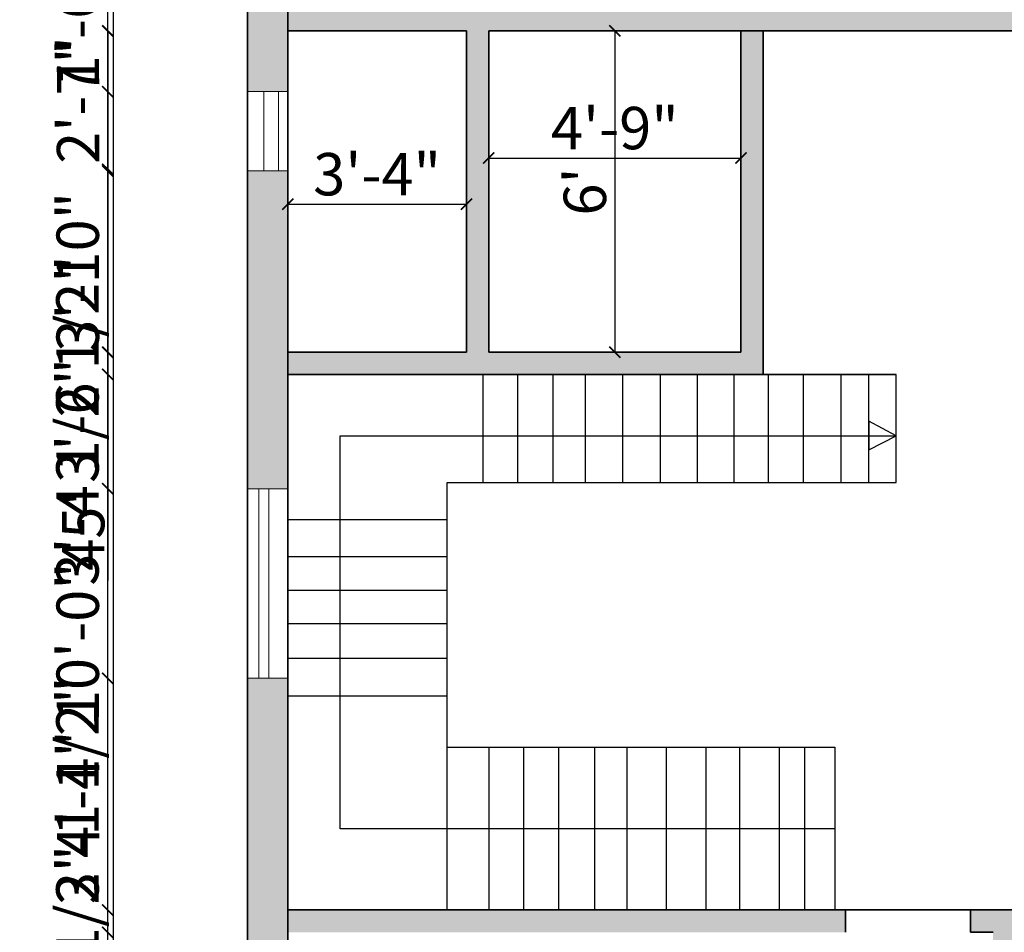
# Model space of a CAD drawing. Units: inches. Extents: x 1704 to 2334, y 1856 to 2559.
# Tile 3 of 10: x 1704 to 1925, y 2148 to 2353. Entities that reach past the tile are written whole.
import ezdxf

# ---------------------------------------------------------------- set-up
doc = ezdxf.new("R2010")
doc.units = ezdxf.units.IN
for name, color, linetype, lineweight in [('A-ANNO-DIMS', 2, 'Continuous', 18), ('A-FLOR-STRS', 7, 'Continuous', 25), ('A-WALL', 7, 'Continuous', 35), ('WINDOW', 6, 'Continuous', 18)]:
    doc.layers.add(name, color=color, linetype=linetype, lineweight=lineweight)
doc.layers.add('A-WALL-PATT', color=18, linetype='Continuous', lineweight=13, true_color=0x000000)
doc.styles.get("Standard").update_dxf_attribs({"font": 'arial.ttf'})
doc.dimstyles.new('ISO-25', dxfattribs={"dimtxt": 9.5, "dimasz": 2.5, "dimexe": 1.25, "dimexo": 0.625, "dimtad": 1, "dimdec": 0, "dimlunit": 4, "dimtxsty": 'Standard', "dimblk": 'ARCHTICK', "dimcen": 2.5, "dimse1": 1, "dimse2": 1, "dimclrd": 3, "dimadec": 0, "dimazin": 0, "dimtfac": 1, "dimtdec": 0, "dimtmove": 0, "dimatfit": 3, "dimfxl": 1, "dimarcsym": 0})

# ---------------------------------------------------------------- blocks, each defined once
blk = doc.blocks.new('_ArchTick')
at = {"color": 0, "linetype": 'ByBlock', "const_width": 0.15}
blk.add_lwpolyline([(-0.5, -0.5), (0.5, 0.5)], dxfattribs=at)
blk = doc.blocks.new('*D15')
at = {"layer": 'A-ANNO-DIMS', "color": 0, "lineweight": -2, "transparency": 16777216}
blk.add_line((1764.01, 2311.2), (1804.01, 2311.2), dxfattribs=at)
at = {"layer": 'Defpoints', "color": 0, "transparency": 16777216}
for p in [(1804.01, 2311.2), (1764.01, 2302.49), (1804.01, 2302.49)]:
    blk.add_point(p, dxfattribs=at)
at = {"layer": 'A-ANNO-DIMS', "color": 0, "lineweight": -2, "transparency": 16777216, "xscale": 2.5, "yscale": 2.5, "zscale": 2.5, "rotation": 180}
blk.add_blockref('_ArchTick', (1764.01, 2311.2), dxfattribs=at)
at = {"layer": 'A-ANNO-DIMS', "color": 0, "lineweight": -2, "transparency": 16777216, "xscale": 2.5, "yscale": 2.5, "zscale": 2.5}
blk.add_blockref('_ArchTick', (1804.01, 2311.2), dxfattribs=at)
at = {"layer": 'A-ANNO-DIMS', "color": 0, "transparency": 16777216, "insert": (1784.01, 2316.68), "char_height": 9.5, "attachment_point": 5}
blk.add_mtext('3\'-4"', dxfattribs=at)
blk = doc.blocks.new('*D16')
at = {"layer": 'A-ANNO-DIMS', "color": 0, "lineweight": -2, "transparency": 16777216}
blk.add_line((1837.26, 2350.04), (1837.26, 2278.04), dxfattribs=at)
at = {"layer": 'Defpoints', "color": 0, "transparency": 16777216}
for p in [(1841.67, 2350.04), (1837.26, 2278.04), (1841.67, 2278.04)]:
    blk.add_point(p, dxfattribs=at)
at = {"layer": 'A-ANNO-DIMS', "color": 0, "lineweight": -2, "transparency": 16777216, "xscale": 2.5, "yscale": 2.5, "zscale": 2.5}
for p, rotation in [((1837.26, 2350.04), 90), ((1837.26, 2278.04), 270)]:
    blk.add_blockref('_ArchTick', p, dxfattribs=dict(at, rotation=rotation))
at = {"layer": 'A-ANNO-DIMS', "color": 0, "transparency": 16777216, "insert": (1831.78, 2314.04), "char_height": 9.5, "attachment_point": 5, "rotation": 90}
blk.add_mtext("6'", dxfattribs=at)
blk = doc.blocks.new('*D17')
at = {"layer": 'A-ANNO-DIMS', "color": 0, "lineweight": -2, "transparency": 16777216}
blk.add_line((1809.01, 2321.54), (1865.51, 2321.54), dxfattribs=at)
at = {"layer": 'Defpoints', "color": 0, "transparency": 16777216}
for p in [(1865.51, 2321.54), (1809.01, 2303.33), (1865.51, 2303.33)]:
    blk.add_point(p, dxfattribs=at)
at = {"layer": 'A-ANNO-DIMS', "color": 0, "lineweight": -2, "transparency": 16777216, "xscale": 2.5, "yscale": 2.5, "zscale": 2.5, "rotation": 180}
blk.add_blockref('_ArchTick', (1809.01, 2321.54), dxfattribs=at)
at = {"layer": 'A-ANNO-DIMS', "color": 0, "lineweight": -2, "transparency": 16777216, "xscale": 2.5, "yscale": 2.5, "zscale": 2.5}
blk.add_blockref('_ArchTick', (1865.51, 2321.54), dxfattribs=at)
at = {"layer": 'A-ANNO-DIMS', "color": 0, "transparency": 16777216, "insert": (1837.26, 2327.02), "char_height": 9.5, "attachment_point": 5}
blk.add_mtext('4\'-9"', dxfattribs=at)
blk = doc.blocks.new('*D23')
at = {"layer": 'A-ANNO-DIMS', "color": 0, "lineweight": -2, "transparency": 16777216}
blk.add_line((1724.87, 2508.04), (1724.87, 1968.04), dxfattribs=at)
at = {"layer": 'Defpoints', "color": 0, "transparency": 16777216}
for p in [(1755.01, 2508.04), (1724.87, 1968.04), (1755.01, 1968.04)]:
    blk.add_point(p, dxfattribs=at)
at = {"layer": 'A-ANNO-DIMS', "color": 0, "lineweight": -2, "transparency": 16777216, "xscale": 2.5, "yscale": 2.5, "zscale": 2.5}
for p, rotation in [((1724.87, 2508.04), 90), ((1724.87, 1968.04), 270)]:
    blk.add_blockref('_ArchTick', p, dxfattribs=dict(at, rotation=rotation))
at = {"layer": 'A-ANNO-DIMS', "color": 0, "transparency": 16777216, "insert": (1719.41, 2238.04), "char_height": 9.5, "attachment_point": 5, "rotation": 90}
blk.add_mtext("45'", dxfattribs=at)
blk = doc.blocks.new('*D37')
at = {"layer": 'A-ANNO-DIMS', "color": 3, "lineweight": -2, "transparency": 16777216}
blk.add_line((1723.66, 1977.04), (1723.66, 2148.04), dxfattribs=at)
at = {"layer": 'Defpoints', "color": 0, "transparency": 16777216}
for p in [(1723.66, 2148.04), (1922.01, 2148.04), (1922.01, 1977.04)]:
    blk.add_point(p, dxfattribs=at)
at = {"layer": 'A-ANNO-DIMS', "color": 3, "lineweight": -2, "transparency": 16777216, "xscale": 2.5, "yscale": 2.5, "zscale": 2.5}
for p, rotation in [((1723.66, 2148.04), 90), ((1723.66, 1977.04), 270)]:
    blk.add_blockref('_ArchTick', p, dxfattribs=dict(at, rotation=rotation))
at = {"layer": 'A-ANNO-DIMS', "color": 0, "transparency": 16777216, "insert": (1718.18, 2062.54), "char_height": 9.5, "attachment_point": 5, "rotation": 90}
blk.add_mtext('14\'-3"', dxfattribs=at)
blk = doc.blocks.new('*D40')
at = {"layer": 'A-ANNO-DIMS', "color": 3, "lineweight": -2, "transparency": 16777216}
blk.add_line((1723.66, 2153.04), (1723.66, 2273.04), dxfattribs=at)
at = {"layer": 'Defpoints', "color": 0, "transparency": 16777216}
for p in [(1723.66, 2273.04), (1764.01, 2273.04), (1764.01, 2153.04)]:
    blk.add_point(p, dxfattribs=at)
at = {"layer": 'A-ANNO-DIMS', "color": 3, "lineweight": -2, "transparency": 16777216, "xscale": 2.5, "yscale": 2.5, "zscale": 2.5}
for p, rotation in [((1723.66, 2273.04), 90), ((1723.66, 2153.04), 270)]:
    blk.add_blockref('_ArchTick', p, dxfattribs=dict(at, rotation=rotation))
at = {"layer": 'A-ANNO-DIMS', "color": 0, "transparency": 16777216, "insert": (1718.18, 2213.04), "char_height": 9.5, "attachment_point": 5, "rotation": 90}
blk.add_mtext('10\'-0"', dxfattribs=at)
blk = doc.blocks.new('*D41')
at = {"layer": 'A-ANNO-DIMS', "color": 3, "lineweight": -2, "transparency": 16777216}
blk.add_line((1764.01, 1864.5), (1900.32, 1864.5), dxfattribs=at)
at = {"layer": 'Defpoints', "color": 0, "transparency": 16777216}
for p in [(1900.32, 2248.82), (1764.01, 2247.44), (1900.32, 1864.5)]:
    blk.add_point(p, dxfattribs=at)
at = {"layer": 'A-ANNO-DIMS', "color": 3, "lineweight": -2, "transparency": 16777216, "xscale": 2.5, "yscale": 2.5, "zscale": 2.5, "rotation": 180}
blk.add_blockref('_ArchTick', (1764.01, 1864.5), dxfattribs=at)
at = {"layer": 'A-ANNO-DIMS', "color": 3, "lineweight": -2, "transparency": 16777216, "xscale": 2.5, "yscale": 2.5, "zscale": 2.5}
blk.add_blockref('_ArchTick', (1900.32, 1864.5), dxfattribs=at)
at = {"layer": 'A-ANNO-DIMS', "color": 0, "transparency": 16777216, "insert": (1832.16, 1870.04), "char_height": 9.5, "attachment_point": 5}
blk.add_mtext('11\'-4 1/2"', dxfattribs=at)
blk = doc.blocks.new('*D43')
at = {"layer": 'A-ANNO-DIMS', "color": 3, "lineweight": -2, "transparency": 16777216}
blk.add_line((1764.01, 2539.39), (1796.13, 2539.39), dxfattribs=at)
at = {"layer": 'Defpoints', "color": 0, "transparency": 16777216}
for p in [(1796.13, 2539.39), (1764.01, 2148.04), (1796.13, 2148.04)]:
    blk.add_point(p, dxfattribs=at)
at = {"layer": 'A-ANNO-DIMS', "color": 3, "lineweight": -2, "transparency": 16777216, "xscale": 2.5, "yscale": 2.5, "zscale": 2.5, "rotation": 180}
blk.add_blockref('_ArchTick', (1764.01, 2539.39), dxfattribs=at)
at = {"layer": 'A-ANNO-DIMS', "color": 3, "lineweight": -2, "transparency": 16777216, "xscale": 2.5, "yscale": 2.5, "zscale": 2.5}
blk.add_blockref('_ArchTick', (1796.13, 2539.39), dxfattribs=at)
at = {"layer": 'A-ANNO-DIMS', "color": 0, "transparency": 16777216, "insert": (1780.07, 2544.86), "char_height": 9.5, "attachment_point": 5}
blk.add_mtext('2\'-8"', dxfattribs=at)
blk = doc.blocks.new('*D46')
at = {"layer": 'A-ANNO-DIMS', "color": 3, "lineweight": -2, "transparency": 16777216}
for p, q in [((2206.36, 2189.49), (2206.36, 2240.62)), ((2206.36, 2153.04), (2206.36, 2189.49))]:
    blk.add_line(p, q, dxfattribs=at)
at = {"layer": 'Defpoints', "color": 0, "transparency": 16777216}
for p in [(1886.55, 2189.49), (2206.36, 2189.49), (1886.55, 2153.04)]:
    blk.add_point(p, dxfattribs=at)
at = {"layer": 'A-ANNO-DIMS', "color": 3, "lineweight": -2, "transparency": 16777216, "xscale": 2.5, "yscale": 2.5, "zscale": 2.5}
for p, rotation in [((2206.36, 2189.49), 90), ((2206.36, 2153.04), 270)]:
    blk.add_blockref('_ArchTick', p, dxfattribs=dict(at, rotation=rotation))
at = {"layer": 'A-ANNO-DIMS', "color": 0, "transparency": 16777216, "insert": (2200.82, 2216.3), "char_height": 9.5, "attachment_point": 5, "rotation": 90}
blk.add_mtext('3\'-0 1/2"', dxfattribs=at)
blk = doc.blocks.new('*D47')
at = {"layer": 'A-ANNO-DIMS', "color": 3, "lineweight": -2, "transparency": 16777216}
for p, q in [((2206.36, 2273.04), (2206.36, 2302.2)), ((2206.36, 2248.82), (2206.36, 2273.04))]:
    blk.add_line(p, q, dxfattribs=at)
at = {"layer": 'Defpoints', "color": 0, "transparency": 16777216}
for p in [(1900.32, 2273.04), (2206.36, 2273.04), (1900.32, 2248.82)]:
    blk.add_point(p, dxfattribs=at)
at = {"layer": 'A-ANNO-DIMS', "color": 3, "lineweight": -2, "transparency": 16777216, "xscale": 2.5, "yscale": 2.5, "zscale": 2.5}
for p, rotation in [((2206.36, 2273.04), 90), ((2206.36, 2248.82), 270)]:
    blk.add_blockref('_ArchTick', p, dxfattribs=dict(at, rotation=rotation))
at = {"layer": 'A-ANNO-DIMS', "color": 0, "transparency": 16777216, "insert": (2200.88, 2288.87), "char_height": 9.5, "attachment_point": 5, "rotation": 90}
blk.add_mtext('2\'-0"', dxfattribs=at)
blk = doc.blocks.new('*D48')
at = {"layer": 'A-ANNO-DIMS', "color": 3, "lineweight": -2, "transparency": 16777216}
for p, q in [((1764.01, 2539.39), (1799.73, 2539.39)), ((1799.73, 2539.39), (1858.41, 2539.39))]:
    blk.add_line(p, q, dxfattribs=at)
at = {"layer": 'Defpoints', "color": 0, "transparency": 16777216}
for p in [(1799.73, 2539.39), (1764.01, 2200.93), (1799.73, 2200.93)]:
    blk.add_point(p, dxfattribs=at)
at = {"layer": 'A-ANNO-DIMS', "color": 3, "lineweight": -2, "transparency": 16777216, "xscale": 2.5, "yscale": 2.5, "zscale": 2.5, "rotation": 180}
blk.add_blockref('_ArchTick', (1764.01, 2539.39), dxfattribs=at)
at = {"layer": 'A-ANNO-DIMS', "color": 3, "lineweight": -2, "transparency": 16777216, "xscale": 2.5, "yscale": 2.5, "zscale": 2.5}
blk.add_blockref('_ArchTick', (1799.73, 2539.39), dxfattribs=at)
at = {"layer": 'A-ANNO-DIMS', "color": 0, "transparency": 16777216, "insert": (1830.32, 2544.93), "char_height": 9.5, "attachment_point": 5}
blk.add_mtext('2\'-11 1/2"', dxfattribs=at)
blk = doc.blocks.new('*D53')
at = {"layer": 'A-ANNO-DIMS', "color": 3, "lineweight": -2, "transparency": 16777216}
for p, q in [((1764.01, 1864.5), (1798.75, 1864.5)), ((1798.75, 1864.5), (1857.43, 1864.5))]:
    blk.add_line(p, q, dxfattribs=at)
at = {"layer": 'Defpoints', "color": 0, "transparency": 16777216}
for p in [(1764.01, 2499.04), (1798.75, 2499.04), (1798.75, 1864.5)]:
    blk.add_point(p, dxfattribs=at)
at = {"layer": 'A-ANNO-DIMS', "color": 3, "lineweight": -2, "transparency": 16777216, "xscale": 2.5, "yscale": 2.5, "zscale": 2.5, "rotation": 180}
blk.add_blockref('_ArchTick', (1764.01, 1864.5), dxfattribs=at)
at = {"layer": 'A-ANNO-DIMS', "color": 3, "lineweight": -2, "transparency": 16777216, "xscale": 2.5, "yscale": 2.5, "zscale": 2.5}
blk.add_blockref('_ArchTick', (1798.75, 1864.5), dxfattribs=at)
at = {"layer": 'A-ANNO-DIMS', "color": 0, "transparency": 16777216, "insert": (1829.34, 1870.04), "char_height": 9.5, "attachment_point": 5}
blk.add_mtext('2\'-10 1/2"', dxfattribs=at)
blk = doc.blocks.new('*D59')
at = {"layer": 'A-ANNO-DIMS', "color": 3, "lineweight": -2, "transparency": 16777216}
for p, q in [((1723.66, 2115.31), (1723.66, 2166.44)), ((1723.66, 2076.84), (1723.66, 2115.31))]:
    blk.add_line(p, q, dxfattribs=at)
at = {"layer": 'Defpoints', "color": 0, "transparency": 16777216}
for p in [(1723.66, 2115.31), (1755.01, 2115.31), (1755.01, 2076.84)]:
    blk.add_point(p, dxfattribs=at)
at = {"layer": 'A-ANNO-DIMS', "color": 3, "lineweight": -2, "transparency": 16777216, "xscale": 2.5, "yscale": 2.5, "zscale": 2.5}
for p, rotation in [((1723.66, 2115.31), 90), ((1723.66, 2076.84), 270)]:
    blk.add_blockref('_ArchTick', p, dxfattribs=dict(at, rotation=rotation))
at = {"layer": 'A-ANNO-DIMS', "color": 0, "transparency": 16777216, "insert": (1718.12, 2142.12), "char_height": 9.5, "attachment_point": 5, "rotation": 90}
blk.add_mtext('3\'-2 1/2"', dxfattribs=at)
blk = doc.blocks.new('*D60')
at = {"layer": 'A-ANNO-DIMS', "color": 3, "lineweight": -2, "transparency": 16777216}
for p, q in [((1723.66, 2153.04), (1723.66, 2204.17)), ((1723.66, 2115.31), (1723.66, 2153.04))]:
    blk.add_line(p, q, dxfattribs=at)
at = {"layer": 'Defpoints', "color": 0, "transparency": 16777216}
for p in [(1723.66, 2153.04), (1764.01, 2153.04), (1755.01, 2115.31)]:
    blk.add_point(p, dxfattribs=at)
at = {"layer": 'A-ANNO-DIMS', "color": 3, "lineweight": -2, "transparency": 16777216, "xscale": 2.5, "yscale": 2.5, "zscale": 2.5}
for p, rotation in [((1723.66, 2153.04), 90), ((1723.66, 2115.31), 270)]:
    blk.add_blockref('_ArchTick', p, dxfattribs=dict(at, rotation=rotation))
at = {"layer": 'A-ANNO-DIMS', "color": 0, "transparency": 16777216, "insert": (1718.12, 2179.86), "char_height": 9.5, "attachment_point": 5, "rotation": 90}
blk.add_mtext('3\'-1 1/2"', dxfattribs=at)
blk = doc.blocks.new('*D62')
at = {"layer": 'A-ANNO-DIMS', "color": 3, "lineweight": -2, "transparency": 16777216}
blk.add_line((1794.77, 2539.39), (1857.04, 2539.39), dxfattribs=at)
at = {"layer": 'Defpoints', "color": 0, "transparency": 16777216}
for p in [(1857.04, 2539.39), (1794.77, 1977.04), (1857.04, 1977.04)]:
    blk.add_point(p, dxfattribs=at)
at = {"layer": 'A-ANNO-DIMS', "color": 3, "lineweight": -2, "transparency": 16777216, "xscale": 2.5, "yscale": 2.5, "zscale": 2.5, "rotation": 180}
blk.add_blockref('_ArchTick', (1794.77, 2539.39), dxfattribs=at)
at = {"layer": 'A-ANNO-DIMS', "color": 3, "lineweight": -2, "transparency": 16777216, "xscale": 2.5, "yscale": 2.5, "zscale": 2.5}
blk.add_blockref('_ArchTick', (1857.04, 2539.39), dxfattribs=at)
at = {"layer": 'A-ANNO-DIMS', "color": 0, "transparency": 16777216, "insert": (1825.9, 2544.93), "char_height": 9.5, "attachment_point": 5}
blk.add_mtext('5\'-2 1/2"', dxfattribs=at)
blk = doc.blocks.new('*D63')
at = {"layer": 'A-ANNO-DIMS', "color": 3, "lineweight": -2, "transparency": 16777216}
blk.add_line((1888.97, 2539.39), (1916.93, 2539.39), dxfattribs=at)
at = {"layer": 'Defpoints', "color": 0, "transparency": 16777216}
for p in [(1916.93, 2539.39), (1888.97, 2153.04), (1916.93, 2153.04)]:
    blk.add_point(p, dxfattribs=at)
at = {"layer": 'A-ANNO-DIMS', "color": 3, "lineweight": -2, "transparency": 16777216, "xscale": 2.5, "yscale": 2.5, "zscale": 2.5, "rotation": 180}
blk.add_blockref('_ArchTick', (1888.97, 2539.39), dxfattribs=at)
at = {"layer": 'A-ANNO-DIMS', "color": 3, "lineweight": -2, "transparency": 16777216, "xscale": 2.5, "yscale": 2.5, "zscale": 2.5}
blk.add_blockref('_ArchTick', (1916.93, 2539.39), dxfattribs=at)
at = {"layer": 'A-ANNO-DIMS', "color": 0, "transparency": 16777216, "insert": (1902.95, 2544.78), "char_height": 9.5, "attachment_point": 5}
blk.add_mtext('2\'-4"', dxfattribs=at)
blk = doc.blocks.new('*D66')
at = {"layer": 'A-ANNO-DIMS', "color": 3, "lineweight": -2, "transparency": 16777216}
for p, q in [((1723.66, 2247.44), (1723.66, 2298.57)), ((1723.66, 2204.96), (1723.66, 2247.44))]:
    blk.add_line(p, q, dxfattribs=at)
at = {"layer": 'Defpoints', "color": 0, "transparency": 16777216}
for p in [(1723.66, 2247.44), (1755.01, 2247.44), (1755.01, 2204.96)]:
    blk.add_point(p, dxfattribs=at)
at = {"layer": 'A-ANNO-DIMS', "color": 3, "lineweight": -2, "transparency": 16777216, "xscale": 2.5, "yscale": 2.5, "zscale": 2.5}
for p, rotation in [((1723.66, 2247.44), 90), ((1723.66, 2204.96), 270)]:
    blk.add_blockref('_ArchTick', p, dxfattribs=dict(at, rotation=rotation))
at = {"layer": 'A-ANNO-DIMS', "color": 0, "transparency": 16777216, "insert": (1718.12, 2274.26), "char_height": 9.5, "attachment_point": 5, "rotation": 90}
blk.add_mtext('3\'-6 1/2"', dxfattribs=at)
blk = doc.blocks.new('*D67')
at = {"layer": 'A-ANNO-DIMS', "color": 3, "lineweight": -2, "transparency": 16777216}
for p, q in [((1723.66, 2336.43), (1723.66, 2364.54)), ((1723.66, 2318.65), (1723.66, 2336.43))]:
    blk.add_line(p, q, dxfattribs=at)
at = {"layer": 'Defpoints', "color": 0, "transparency": 16777216}
for p in [(1723.66, 2336.43), (1755.01, 2336.43), (1755.01, 2318.65)]:
    blk.add_point(p, dxfattribs=at)
at = {"layer": 'A-ANNO-DIMS', "color": 3, "lineweight": -2, "transparency": 16777216, "xscale": 2.5, "yscale": 2.5, "zscale": 2.5}
for p, rotation in [((1723.66, 2336.43), 90), ((1723.66, 2318.65), 270)]:
    blk.add_blockref('_ArchTick', p, dxfattribs=dict(at, rotation=rotation))
at = {"layer": 'A-ANNO-DIMS', "color": 0, "transparency": 16777216, "insert": (1718.18, 2351.73), "char_height": 9.5, "attachment_point": 5, "rotation": 90}
blk.add_mtext('1\'-6"', dxfattribs=at)
blk = doc.blocks.new('*D70')
at = {"layer": 'A-ANNO-DIMS', "color": 3, "lineweight": -2, "transparency": 16777216}
blk.add_line((1799.73, 1864.5), (1886.55, 1864.5), dxfattribs=at)
at = {"layer": 'Defpoints', "color": 0, "transparency": 16777216}
for p in [(1886.55, 2189.49), (1799.73, 2153.04), (1886.55, 1864.5)]:
    blk.add_point(p, dxfattribs=at)
at = {"layer": 'A-ANNO-DIMS', "color": 3, "lineweight": -2, "transparency": 16777216, "xscale": 2.5, "yscale": 2.5, "zscale": 2.5, "rotation": 180}
blk.add_blockref('_ArchTick', (1799.73, 1864.5), dxfattribs=at)
at = {"layer": 'A-ANNO-DIMS', "color": 3, "lineweight": -2, "transparency": 16777216, "xscale": 2.5, "yscale": 2.5, "zscale": 2.5}
blk.add_blockref('_ArchTick', (1886.55, 1864.5), dxfattribs=at)
at = {"layer": 'A-ANNO-DIMS', "color": 0, "transparency": 16777216, "insert": (1843.14, 1869.98), "char_height": 9.5, "attachment_point": 5}
blk.add_mtext('7\'-3"', dxfattribs=at)
blk = doc.blocks.new('*D71')
at = {"layer": 'A-ANNO-DIMS', "color": 3, "lineweight": -2, "transparency": 16777216}
blk.add_line((1723.659742, 2153.039492), (1723.659742, 2204.962868), dxfattribs=at)
at = {"layer": 'Defpoints', "color": 0, "transparency": 16777216}
for p in [(1723.659742, 2204.962868), (1755.009742, 2204.962868), (1764.009742, 2153.039492)]:
    blk.add_point(p, dxfattribs=at)
at = {"layer": 'A-ANNO-DIMS', "color": 3, "lineweight": -2, "transparency": 16777216, "xscale": 2.5, "yscale": 2.5, "zscale": 2.5}
for p, rotation in [((1723.659742, 2204.962868), 90), ((1723.659742, 2153.039492), 270)]:
    blk.add_blockref('_ArchTick', p, dxfattribs=dict(at, rotation=rotation))
at = {"layer": 'A-ANNO-DIMS', "color": 0, "transparency": 16777216, "insert": (1718.284742, 2179.00118), "char_height": 9.5, "attachment_point": 5, "rotation": 90}
blk.add_mtext('4\'-4"', dxfattribs=at)
blk = doc.blocks.new('*D72')
at = {"layer": 'A-ANNO-DIMS', "color": 3, "lineweight": -2, "transparency": 16777216}
for p, q in [((1723.66, 2318.65), (1723.66, 2278.04)), ((1723.66, 2278.04), (1723.66, 2226.91))]:
    blk.add_line(p, q, dxfattribs=at)
at = {"layer": 'Defpoints', "color": 0, "transparency": 16777216}
for p in [(1755.01, 2318.65), (1723.66, 2278.04), (1764.01, 2278.04)]:
    blk.add_point(p, dxfattribs=at)
at = {"layer": 'A-ANNO-DIMS', "color": 3, "lineweight": -2, "transparency": 16777216, "xscale": 2.5, "yscale": 2.5, "zscale": 2.5}
for p, rotation in [((1723.66, 2318.65), 90), ((1723.66, 2278.04), 270)]:
    blk.add_blockref('_ArchTick', p, dxfattribs=dict(at, rotation=rotation))
at = {"layer": 'A-ANNO-DIMS', "color": 0, "transparency": 16777216, "insert": (1718.12, 2251.22), "char_height": 9.5, "attachment_point": 5, "rotation": 90}
blk.add_mtext('3\'-4 1/2"', dxfattribs=at)
blk = doc.blocks.new('*D74')
at = {"layer": 'A-ANNO-DIMS', "color": 3, "lineweight": -2, "transparency": 16777216}
blk.add_line((1916.93, 2539.39), (1948.02, 2539.39), dxfattribs=at)
at = {"layer": 'Defpoints', "color": 0, "transparency": 16777216}
for p in [(1948.02, 2539.39), (1916.93, 2153.04), (1948.02, 2153.04)]:
    blk.add_point(p, dxfattribs=at)
at = {"layer": 'A-ANNO-DIMS', "color": 3, "lineweight": -2, "transparency": 16777216, "xscale": 2.5, "yscale": 2.5, "zscale": 2.5, "rotation": 180}
blk.add_blockref('_ArchTick', (1916.93, 2539.39), dxfattribs=at)
at = {"layer": 'A-ANNO-DIMS', "color": 3, "lineweight": -2, "transparency": 16777216, "xscale": 2.5, "yscale": 2.5, "zscale": 2.5}
blk.add_blockref('_ArchTick', (1948.02, 2539.39), dxfattribs=at)
at = {"layer": 'A-ANNO-DIMS', "color": 0, "transparency": 16777216, "insert": (1932.47, 2544.78), "char_height": 9.5, "attachment_point": 5}
blk.add_mtext('2\'-7"', dxfattribs=at)
blk = doc.blocks.new('*D78')
at = {"layer": 'A-ANNO-DIMS', "color": 3, "lineweight": -2, "transparency": 16777216}
blk.add_line((1723.66, 2273.04), (1723.66, 2319.04), dxfattribs=at)
at = {"layer": 'Defpoints', "color": 0, "transparency": 16777216}
for p in [(1723.66, 2319.04), (1993.01, 2319.04), (1993.01, 2273.04)]:
    blk.add_point(p, dxfattribs=at)
at = {"layer": 'A-ANNO-DIMS', "color": 3, "lineweight": -2, "transparency": 16777216, "xscale": 2.5, "yscale": 2.5, "zscale": 2.5}
for p, rotation in [((1723.66, 2319.04), 90), ((1723.66, 2273.04), 270)]:
    blk.add_blockref('_ArchTick', p, dxfattribs=dict(at, rotation=rotation))
at = {"layer": 'A-ANNO-DIMS', "color": 0, "transparency": 16777216, "insert": (1718.18, 2296.04), "char_height": 9.5, "attachment_point": 5, "rotation": 90}
blk.add_mtext('3\'-10"', dxfattribs=at)
blk = doc.blocks.new('*D79')
at = {"layer": 'A-ANNO-DIMS', "color": 3, "lineweight": -2, "transparency": 16777216}
blk.add_line((1723.66, 2350.04), (1723.66, 2319.04), dxfattribs=at)
at = {"layer": 'Defpoints', "color": 0, "transparency": 16777216}
for p in [(1998.01, 2350.04), (1723.66, 2319.04), (1993.01, 2319.04)]:
    blk.add_point(p, dxfattribs=at)
at = {"layer": 'A-ANNO-DIMS', "color": 3, "lineweight": -2, "transparency": 16777216, "xscale": 2.5, "yscale": 2.5, "zscale": 2.5}
for p, rotation in [((1723.66, 2350.04), 90), ((1723.66, 2319.04), 270)]:
    blk.add_blockref('_ArchTick', p, dxfattribs=dict(at, rotation=rotation))
at = {"layer": 'A-ANNO-DIMS', "color": 0, "transparency": 16777216, "insert": (1718.27, 2334.54), "char_height": 9.5, "attachment_point": 5, "rotation": 90}
blk.add_mtext('2\'-7"', dxfattribs=at)
blk = doc.blocks.new('*D80')
at = {"layer": 'A-ANNO-DIMS', "color": 3, "lineweight": -2, "transparency": 16777216}
blk.add_line((1900.32, 2539.39), (1993.01, 2539.39), dxfattribs=at)
at = {"layer": 'Defpoints', "color": 0, "transparency": 16777216}
for p in [(1993.01, 2539.39), (1900.32, 2273.04), (1993.01, 2273.04)]:
    blk.add_point(p, dxfattribs=at)
at = {"layer": 'A-ANNO-DIMS', "color": 3, "lineweight": -2, "transparency": 16777216, "xscale": 2.5, "yscale": 2.5, "zscale": 2.5, "rotation": 180}
blk.add_blockref('_ArchTick', (1900.32, 2539.39), dxfattribs=at)
at = {"layer": 'A-ANNO-DIMS', "color": 3, "lineweight": -2, "transparency": 16777216, "xscale": 2.5, "yscale": 2.5, "zscale": 2.5}
blk.add_blockref('_ArchTick', (1993.01, 2539.39), dxfattribs=at)
at = {"layer": 'A-ANNO-DIMS', "color": 0, "transparency": 16777216, "insert": (1946.66, 2544.93), "char_height": 9.5, "attachment_point": 5}
blk.add_mtext('7\'-8 1/2"', dxfattribs=at)
blk = doc.blocks.new('*D81')
at = {"layer": 'A-ANNO-DIMS', "color": 3, "lineweight": -2, "transparency": 16777216}
blk.add_line((2206.36, 2074.93), (2206.36, 2148.04), dxfattribs=at)
at = {"layer": 'Defpoints', "color": 0, "transparency": 16777216}
for p in [(1796.13, 2148.04), (2206.36, 2148.04), (1790.01, 2074.93)]:
    blk.add_point(p, dxfattribs=at)
at = {"layer": 'A-ANNO-DIMS', "color": 3, "lineweight": -2, "transparency": 16777216, "xscale": 2.5, "yscale": 2.5, "zscale": 2.5}
for p, rotation in [((2206.36, 2148.04), 90), ((2206.36, 2074.93), 270)]:
    blk.add_blockref('_ArchTick', p, dxfattribs=dict(at, rotation=rotation))
at = {"layer": 'A-ANNO-DIMS', "color": 0, "transparency": 16777216, "insert": (2200.88, 2111.48), "char_height": 9.5, "attachment_point": 5, "rotation": 90}
blk.add_mtext('6\'-1"', dxfattribs=at)

msp = doc.modelspace()

# ---------------------------------------------------------------- hatches: boundary and pattern name
at = {"layer": 'A-WALL-PATT'}
h = msp.add_hatch(color=256, dxfattribs=at)
h.dxf.hatch_style = 1
h.paths.add_polyline_path([(1764.01, 2204.96), (1755.01, 2204.96), (1755.01, 2115.31), (1764.01, 2115.31)])
h.paths.add_polyline_path([(1764.01, 2076.84), (1755.01, 2076.84), (1755.01, 1968.04), (1794.77, 1968.04), (1794.77, 1977.04), (1764.01, 1977.04)])
h.paths.add_polyline_path([(1927.01, 1977.04), (1927.01, 2069.24), (1993.01, 2069.24), (1993.01, 1977.04)], flags=16)
h.paths.add_polyline_path([(1927.01, 2074.24), (1927.01, 2148.04), (1993.01, 2148.04), (1993.01, 2074.24)], flags=16)
h.paths.add_polyline_path([(1764.01, 2318.65), (1755.01, 2318.65), (1755.01, 2247.44), (1764.01, 2247.44)])
h.paths.add_polyline_path([(1764.01, 2499.04), (1798.75, 2499.04), (1798.75, 2508.04), (1755.01, 2508.04), (1755.01, 2336.43), (1764.01, 2336.43)])
h.paths.add_polyline_path([(1950.56, 2508.04), (1847.17, 2508.04), (1847.17, 2499.04), (1950.56, 2499.04)])
h.paths.add_polyline_path([(2059.64, 2508.04), (1975.68, 2508.04), (1975.68, 2499.04), (2059.64, 2499.04)])
h.paths.add_polyline_path([(2175.01, 2508.04), (2108.25, 2508.04), (2108.25, 2499.04), (2166.01, 2499.04), (2166.01, 1977.04), (2166.01, 1972.26), (2166.01, 1968.04), (2175.01, 1968.04)])
h.paths.add_polyline_path([(2166.01, 2319.04), (1993.01, 2319.04), (1993.01, 2273.04), (1998.01, 2273.04), (1998.01, 2314.04), (2166.01, 2314.04)])
h.paths.add_polyline_path([(2054.53, 2117.04), (1998.01, 2117.04), (1998.01, 2112.04), (2054.53, 2112.04)])
h.paths.add_polyline_path([(2166.01, 2117.04), (2105.53, 2117.04), (2105.53, 2112.04), (2166.01, 2112.04)])
h.paths.add_polyline_path([(1927.01, 2499.04), (1922.01, 2499.04), (1922.01, 2355.04), (1764.01, 2355.04), (1764.01, 2350.04), (1804.01, 2350.04), (1804.01, 2278.04), (1764.01, 2278.04), (1764.01, 2273.04), (1870.51, 2273.04), (1870.51, 2278.04), (1870.51, 2350.04), (1865.51, 2350.04), (1865.51, 2278.04), (1809.01, 2278.04), (1809.01, 2350.04), (1922.01, 2350.04), (1927.01, 2350.04), (1998.01, 2350.04), (1998.01, 2499.04), (1993.01, 2499.04), (1993.01, 2355.04), (1927.01, 2355.04)])
h.paths.add_polyline_path([(2131.1, 2203.36), (2144.85, 2203.36), (2144.85, 2212.38), (2131.1, 2212.38)], flags=25)
h.paths.add_polyline_path([(2010.94, 2265.21), (2036.85, 2265.21), (2036.85, 2274.23), (2010.94, 2274.23)], flags=9)
h.paths.add_polyline_path([(2010.9, 2274.71), (2056.95, 2274.71), (2056.95, 2284.04), (2010.9, 2284.04)], flags=25)
h.paths.add_polyline_path([(2003.27, 2440.18), (2049.79, 2440.18), (2049.79, 2449.51), (2003.27, 2449.51)], flags=9)
h.paths.add_polyline_path([(1934.96, 2428.22), (1967.48, 2428.22), (1967.48, 2437.55), (1934.96, 2437.55)], flags=25)
h.paths.add_polyline_path([(1778.93, 2466.23), (1827.79, 2466.23), (1827.79, 2475.56), (1778.93, 2475.56)], flags=25)
h.paths.add_polyline_path([(1938.32, 2043.05), (1970.37, 2043.05), (1970.37, 2052.39), (1938.32, 2052.39)], flags=8)
h.paths.add_polyline_path([(1932.21, 2095.38), (1956.75, 2095.38), (1956.75, 2104.56), (1932.21, 2104.56)], flags=8)
h.paths.add_polyline_path([(1888.97, 2148.04), (1888.97, 2153.04), (1764.01, 2153.04), (1764.01, 2148.04)])
h.paths.add_polyline_path([(1922.01, 2059.61), (1927.01, 2059.61), (1927.01, 2044.47), (1922.01, 2044.47), (1922.01, 1977.04), (1857.04, 1977.04), (1857.04, 1968.04), (1998.01, 1968.04), (1998.01, 1977.04), (1998.01, 2153.04), (1916.93, 2153.04), (1916.93, 2148.04), (1922.01, 2148.04)])

# ---------------------------------------------------------------- linework, layer by layer
at = {"layer": 'A-FLOR-STRS'}
for p, q in [((1807.77, 2248.82), (1807.77, 2273.04)), ((1815.53, 2248.82), (1815.53, 2273.04)), ((1823.43, 2248.82), (1823.43, 2273.04)), ((1830.66, 2248.82), (1830.66, 2273.04)), ((1839.05, 2248.82), (1839.05, 2273.04)), ((1847.46, 2248.82), (1847.46, 2273.04)), ((1855.77, 2248.82), (1855.77, 2273.04)), ((1864.02, 2248.82), (1864.02, 2273.04)), ((1871.71, 2248.82), (1871.71, 2273.04)), ((1879.5, 2248.82), (1879.5, 2273.04)), ((1887.99, 2248.82), (1887.99, 2273.04)), ((1894.19, 2248.82), (1894.19, 2273.04)), ((1900.32, 2248.82), (1900.32, 2273.04)), ((1900.32, 2259.26), (1894.19, 2262.56)), ((1894.19, 2262.56), (1894.19, 2256.16)), ((1775.76, 2171.26), (1775.76, 2259.26)), ((1775.76, 2259.26), (1900.32, 2259.26)), ((1894.19, 2256.16), (1900.32, 2259.26)), ((1799.73, 2153.04), (1799.73, 2248.82)), ((1799.73, 2248.82), (1900.32, 2248.82)), ((1799.73, 2240.5), (1764.01, 2240.5)), ((1799.73, 2232.18), (1764.01, 2232.18)), ((1799.73, 2224.66), (1764.01, 2224.66)), ((1799.73, 2217.14), (1764.01, 2217.14)), ((1799.73, 2209.36), (1764.01, 2209.36)), ((1799.73, 2200.93), (1764.01, 2200.93)), ((1799.73, 2153.04), (1799.73, 2189.49)), ((1799.73, 2189.49), (1886.55, 2189.49)), ((1809.11, 2153.04), (1809.11, 2189.49)), ((1816.9, 2153.04), (1816.9, 2189.49)), ((1824.69, 2153.04), (1824.69, 2189.49)), ((1832.75, 2153.04), (1832.75, 2189.49)), ((1840, 2153.04), (1840, 2189.49)), ((1848.87, 2153.04), (1848.87, 2189.49)), ((1857.73, 2153.04), (1857.73, 2189.49)), ((1865.25, 2153.04), (1865.25, 2189.49)), ((1874.12, 2153.04), (1874.12, 2189.49)), ((1879.83, 2153.04), (1879.83, 2189.49)), ((1886.55, 2189.49), (1886.55, 2153.04)), ((1886.55, 2171.26), (1775.76, 2171.26)), ((1764.01, 2153.04), (1799.73, 2153.04))]:
    msp.add_line(p, q, dxfattribs=at)
at = {"layer": 'A-WALL'}
for p, q in [((1764.01, 1977.04), (1764.01, 2499.04)), ((1764.01, 2350.04), (1804.01, 2350.04)), ((1804.01, 2278.04), (1804.01, 2350.04)), ((1809.01, 2278.04), (1809.01, 2350.04)), ((1809.01, 2350.04), (1922.01, 2350.04)), ((1865.51, 2278.04), (1865.51, 2350.04)), ((1870.51, 2278.04), (1870.51, 2350.04)), ((1927.01, 2350.04), (1922.01, 2350.04)), ((1764.01, 2278.04), (1804.01, 2278.04)), ((1809.01, 2278.04), (1865.51, 2278.04)), ((1870.51, 2278.04), (1870.51, 2273.04)), ((1764.01, 2273.04), (1900.32, 2273.04)), ((1764.01, 2153.04), (1948.02, 2153.04)), ((1888.97, 2153.04), (1888.97, 2148.04)), ((1916.93, 2153.04), (1916.93, 2148.04)), ((1916.93, 2148.04), (1922.01, 2148.04))]:
    msp.add_line(p, q, dxfattribs=at)
msp.add_lwpolyline([(1998.01, 1968.04), (1755.01, 1968.04), (1755.01, 2508.04), (2175.01, 2508.04), (2175.01, 1968.04), (2166.01, 1968.04)], dxfattribs=at)
at = {"layer": 'WINDOW'}
for p, q in [((1764.01, 2336.43), (1755.01, 2336.43)), ((1755.01, 2336.43), (1755.01, 2318.65)), ((1758.63, 2318.65), (1758.63, 2336.43)), ((1761.96, 2318.65), (1761.96, 2336.43)), ((1764.01, 2318.65), (1764.01, 2336.43)), ((1755.01, 2318.65), (1764.01, 2318.65)), ((1764.01, 2247.44), (1755.01, 2247.44)), ((1755.01, 2247.44), (1755.01, 2204.96)), ((1757.51, 2204.96), (1757.51, 2247.44)), ((1759.77, 2204.96), (1759.77, 2247.44)), ((1764.01, 2204.96), (1764.01, 2247.44)), ((1755.01, 2204.96), (1764.01, 2204.96))]:
    msp.add_line(p, q, dxfattribs=at)

# ---------------------------------------------------------------- dimensions: what is measured, and where the dimension line sits
at = {"layer": 'A-ANNO-DIMS'}
for base, p1, p2, override, picture, middle in [((1799.73, 2539.39), (1764.01, 2200.93), (1799.73, 2200.93), {"dimdec": 1, "dimlfac": 1, "dimrnd": 0, "dimzin": 1, "dimdsep": 46, "dimlunit": 4, "dimfrac": 2}, '*D48', (1830.32, 2544.93)), ((1857.04, 2539.39), (1794.77, 1977.04), (1857.04, 1977.04), {"dimdec": 1, "dimlfac": 1, "dimrnd": 0, "dimzin": 1, "dimdsep": 46, "dimlunit": 4, "dimfrac": 2}, '*D62', (1825.9, 2544.93)), ((1993.01, 2539.39), (1900.32, 2273.04), (1993.01, 2273.04), {"dimdec": 1, "dimlfac": 1, "dimrnd": 0, "dimzin": 1, "dimdsep": 46, "dimlunit": 4, "dimfrac": 2}, '*D80', (1946.66, 2544.93)), ((1796.13, 2539.39), (1764.01, 2148.04), (1796.13, 2148.04), {"dimdec": 1, "dimlfac": 1, "dimrnd": 0, "dimzin": 1, "dimdsep": 46, "dimlunit": 4, "dimfrac": 2}, '*D43', (1780.07, 2544.86)), ((1916.93, 2539.39), (1888.97, 2153.04), (1916.93, 2153.04), {"dimdec": 1, "dimlfac": 1, "dimrnd": 0, "dimzin": 1, "dimdsep": 46, "dimlunit": 4, "dimfrac": 2}, '*D63', (1902.95, 2544.78)), ((1948.02, 2539.39), (1916.93, 2153.04), (1948.02, 2153.04), {"dimdec": 1, "dimlfac": 1, "dimrnd": 0, "dimzin": 1, "dimdsep": 46, "dimlunit": 4, "dimfrac": 2}, '*D74', (1932.47, 2544.78)), ((1798.75, 1864.5), (1764.01, 2499.04), (1798.75, 2499.04), {"dimdec": 1, "dimlfac": 1, "dimrnd": 0, "dimzin": 1, "dimdsep": 46, "dimlunit": 4, "dimfrac": 2}, '*D53', (1829.34, 1870.04)), ((1865.50974237, 2321.54056966), (1809.00974237, 2303.32817591), (1865.50974237, 2303.32817591), {"dimclrd": 0, "dimclre": 0, "dimclrt": 0}, '*D17', (1837.25974237, 2327.01601304)), ((1804.01, 2311.2), (1764.01, 2302.49), (1804.01, 2302.49), {"dimclrd": 0, "dimclre": 0, "dimclrt": 0}, '*D15', (1784.01, 2316.68)), ((1900.32, 1864.5), (1764.01, 2247.44), (1900.32, 2248.82), {"dimdec": 1, "dimlfac": 1, "dimrnd": 0, "dimzin": 1, "dimdsep": 46, "dimlunit": 4, "dimfrac": 2}, '*D41', (1832.16, 1870.04)), ((1886.55, 1864.5), (1799.73, 2153.04), (1886.55, 2189.49), {"dimdec": 1, "dimlfac": 1, "dimrnd": 0, "dimzin": 1, "dimdsep": 46, "dimlunit": 4, "dimfrac": 2}, '*D70', (1843.14, 1869.98))]:
    dim = msp.add_linear_dim(base=base, p1=p1, p2=p2, dimstyle='ISO-25', override=override, dxfattribs=at)
    dim.commit()
    dim.dimension.update_dxf_attribs({"geometry": picture, "text_midpoint": middle})
for base, p1, p2, override, picture, middle in [((1724.87, 1968.04), (1755.01, 2508.04), (1755.01, 1968.04), {"dimclrd": 0, "dimclre": 0, "dimclrt": 0}, '*D23', (1719.41, 2238.04)), ((1723.66, 2336.43), (1755.01, 2318.65), (1755.01, 2336.43), {"dimdec": 1, "dimlfac": 1, "dimrnd": 0, "dimzin": 1, "dimdsep": 46, "dimlunit": 4, "dimfrac": 2}, '*D67', (1718.18, 2351.73)), ((1723.66, 2319.04), (1998.01, 2350.04), (1993.01, 2319.04), {"dimdec": 1, "dimlfac": 1, "dimrnd": 0, "dimzin": 1, "dimdsep": 46, "dimlunit": 4, "dimfrac": 2}, '*D79', (1718.27, 2334.54)), ((1837.26, 2278.04), (1841.67, 2350.04), (1841.67, 2278.04), {"dimclrd": 0, "dimclre": 0, "dimclrt": 0}, '*D16', (1831.78, 2314.04)), ((1723.66, 2319.04), (1993.01, 2273.04), (1993.01, 2319.04), {"dimdec": 1, "dimlfac": 1, "dimrnd": 0, "dimzin": 1, "dimdsep": 46, "dimlunit": 4, "dimfrac": 2}, '*D78', (1718.18, 2296.04)), ((1723.66, 2278.04), (1755.01, 2318.65), (1764.01, 2278.04), {"dimdec": 1, "dimlfac": 1, "dimrnd": 0, "dimzin": 1, "dimdsep": 46, "dimlunit": 4, "dimfrac": 2}, '*D72', (1718.12, 2251.22)), ((2206.36, 2273.04), (1900.32, 2248.82), (1900.32, 2273.04), {"dimdec": 1, "dimlfac": 1, "dimrnd": 0, "dimzin": 1, "dimdsep": 46, "dimlunit": 4, "dimfrac": 2}, '*D47', (2200.88, 2288.87)), ((1723.66, 2247.44), (1755.01, 2204.96), (1755.01, 2247.44), {"dimdec": 1, "dimlfac": 1, "dimrnd": 0, "dimzin": 1, "dimdsep": 46, "dimlunit": 4, "dimfrac": 2}, '*D66', (1718.12, 2274.26)), ((1723.66, 2273.04), (1764.01, 2153.04), (1764.01, 2273.04), {"dimdec": 1, "dimlfac": 1, "dimrnd": 0, "dimzin": 1, "dimdsep": 46, "dimlunit": 4, "dimfrac": 2}, '*D40', (1718.18, 2213.04)), ((2206.3597, 2189.4875), (1886.552, 2153.0395), (1886.552, 2189.4875), {"dimdec": 1, "dimlfac": 1, "dimrnd": 0, "dimzin": 1, "dimdsep": 46, "dimlunit": 4, "dimfrac": 2}, '*D46', (2200.8195, 2216.3042)), ((1723.66, 2204.96), (1764.01, 2153.04), (1755.01, 2204.96), {"dimdec": 1, "dimlfac": 1, "dimrnd": 0, "dimzin": 1, "dimdsep": 46, "dimlunit": 4, "dimfrac": 2}, '*D71', (1718.28, 2179)), ((1723.66, 2153.04), (1755.01, 2115.31), (1764.01, 2153.04), {"dimdec": 1, "dimlfac": 1, "dimrnd": 0, "dimzin": 1, "dimdsep": 46, "dimlunit": 4, "dimfrac": 2}, '*D60', (1718.12, 2179.86)), ((1723.66, 2115.31), (1755.01, 2076.84), (1755.01, 2115.31), {"dimdec": 1, "dimlfac": 1, "dimrnd": 0, "dimzin": 1, "dimdsep": 46, "dimlunit": 4, "dimfrac": 2}, '*D59', (1718.12, 2142.12)), ((1723.66, 2148.04), (1922.01, 1977.04), (1922.01, 2148.04), {"dimdec": 1, "dimlfac": 1, "dimrnd": 0, "dimzin": 1, "dimdsep": 46, "dimlunit": 4, "dimfrac": 2}, '*D37', (1718.18, 2062.54)), ((2206.36, 2148.04), (1790.01, 2074.93), (1796.13, 2148.04), {"dimdec": 1, "dimlfac": 1, "dimrnd": 0, "dimzin": 1, "dimdsep": 46, "dimlunit": 4, "dimfrac": 2}, '*D81', (2200.88, 2111.48))]:
    dim = msp.add_linear_dim(base=base, p1=p1, p2=p2, angle=90, dimstyle='ISO-25', override=override, dxfattribs=at)
    dim.commit()
    dim.dimension.update_dxf_attribs({"geometry": picture, "text_midpoint": middle})

doc.saveas('drawing.dxf')
